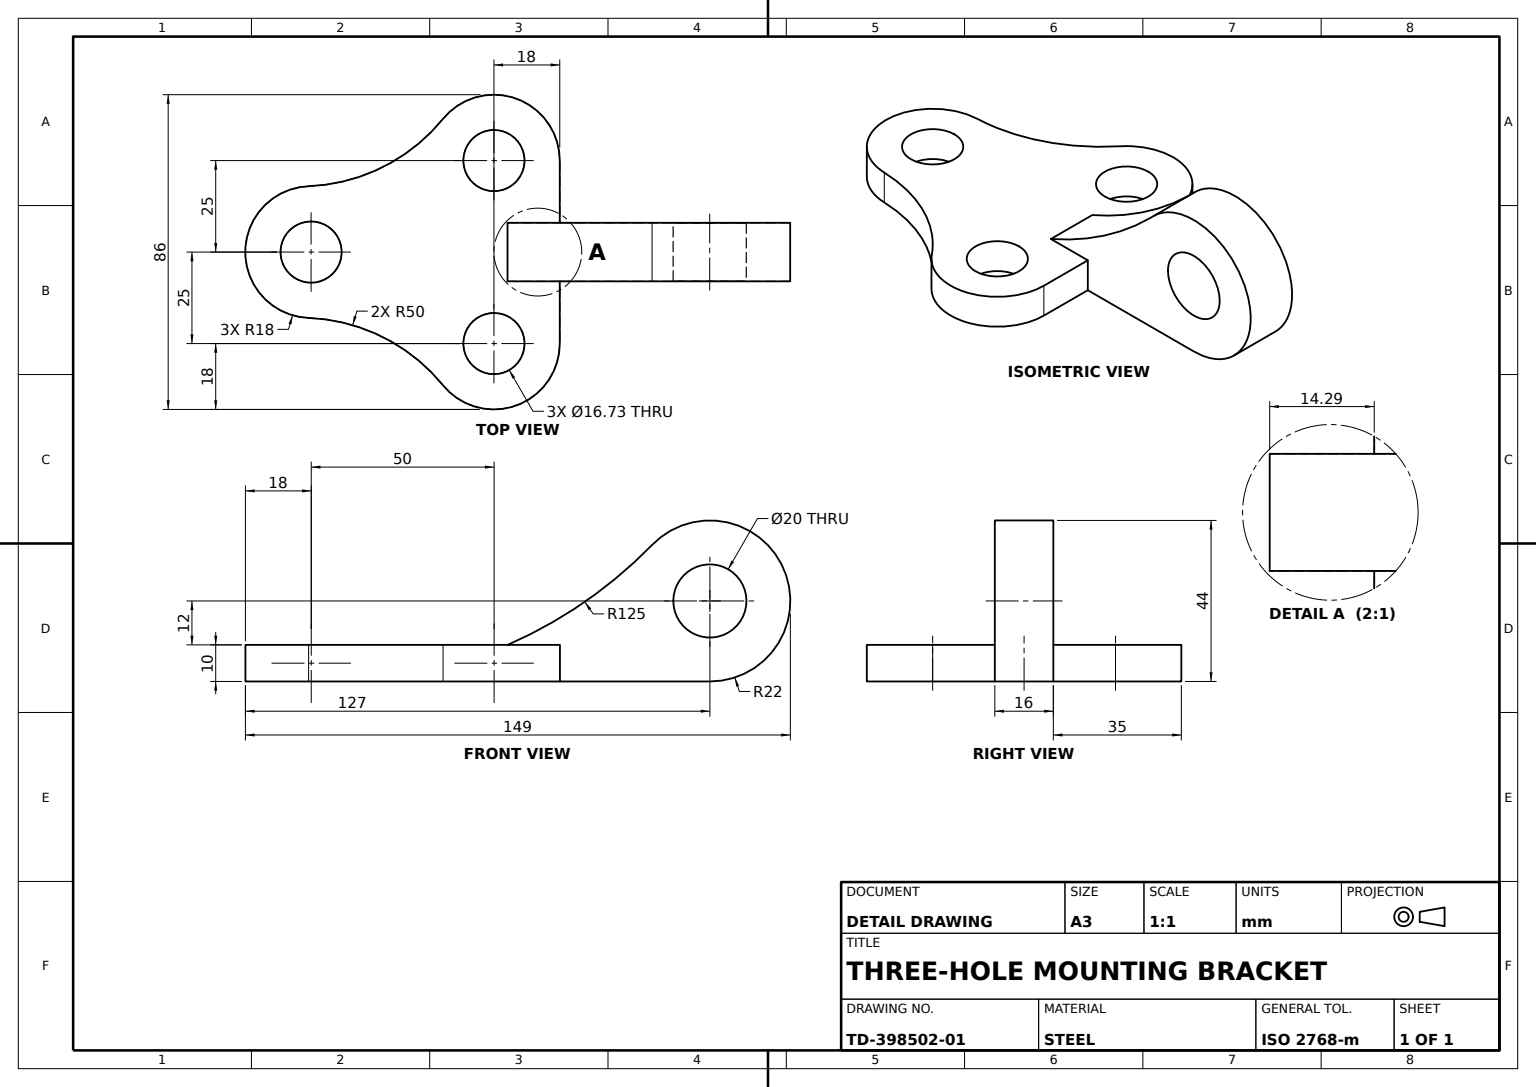
SolidWorks part; units mm, degrees
material "Plain Carbon Steel"
ref_plane "Front Plane" through (0, 0, 0) normal (0, 0, 1) x (1, 0, 0)
ref_plane "Top Plane" through (0, 0, 0) normal (0, 1, 0) x (1, 0, 0)
ref_plane "Right Plane" through (0, 0, 0) normal (1, 0, 0) x (0, 0, -1)
sketch "Base Plate Profile Sketch" plane through (0, 0, 0) normal (0, 1, 0) x (1, 0, 0)
  line L0 (-83.4781, 0) -> (166.7404, 0) construction
  line L1 (68, 25) -> (68, -25)
  circle A6 centre (0, 0) radius 8.3639
  arc A7 (-0.7207, 17.9856) -> (-0.7207, -17.9856) centre (0, 0) ccw
  circle A8 centre (50, 25) radius 8.3639
  arc A9 (68, 25) -> (36.044, 36.3679) centre (50, 25) ccw
  arc A10 (-0.7207, 17.9856) -> (36.044, 36.3679) centre (-2.7227, 67.9455) ccw
  arc A11 (-0.7207, -17.9856) -> (36.044, -36.3679) centre (-2.7227, -67.9455) cw
  arc A12 (68, -25) -> (36.044, -36.3679) centre (50, -25) cw
  circle A13 centre (50, -25) radius 8.3639
  dimension "D1" = 16.7279
  dimension "D2" = 36
  dimension "D3" = 25
  dimension "D4" = 50
  dimension "D5" = 50
extrude "Base Plate 3-Hole" add sketch "Base Plate Profile Sketch" along normal blind 10
sketch "Bored Lug Profile Sketch" plane through (0, 0, 0) normal (0, 0, 1) x (1, 0, 0)
  line L0 (68, 10) -> (36.044, 10) construction
  line L1 (68, 10) -> (68, 0) construction
  line L2 (68, 10) -> (53.71, 10)
  line L3 (68, 10) -> (68, 0)
  line L4 (68, 0) -> (109, 0)
  line L5 (36.044, 0) -> (68, 0) construction
  arc A0 (109, 0) -> (93.2379, 37.3479) centre (109, 22) ccw
  circle A1 centre (109, 22) radius 10
  arc A2 (53.71, 10) -> (93.2379, 37.3479) centre (3.6806, 124.5515) ccw
  dimension "D1" = 20
  dimension "D2" = 44
  dimension "D5" = 125
  dimension "D6" = 14.29
  dimension "D3" = 41
  dimension "D4" = 22
extrude "Bored Lug" add sketch "Bored Lug Profile Sketch" along normal mid plane 16
